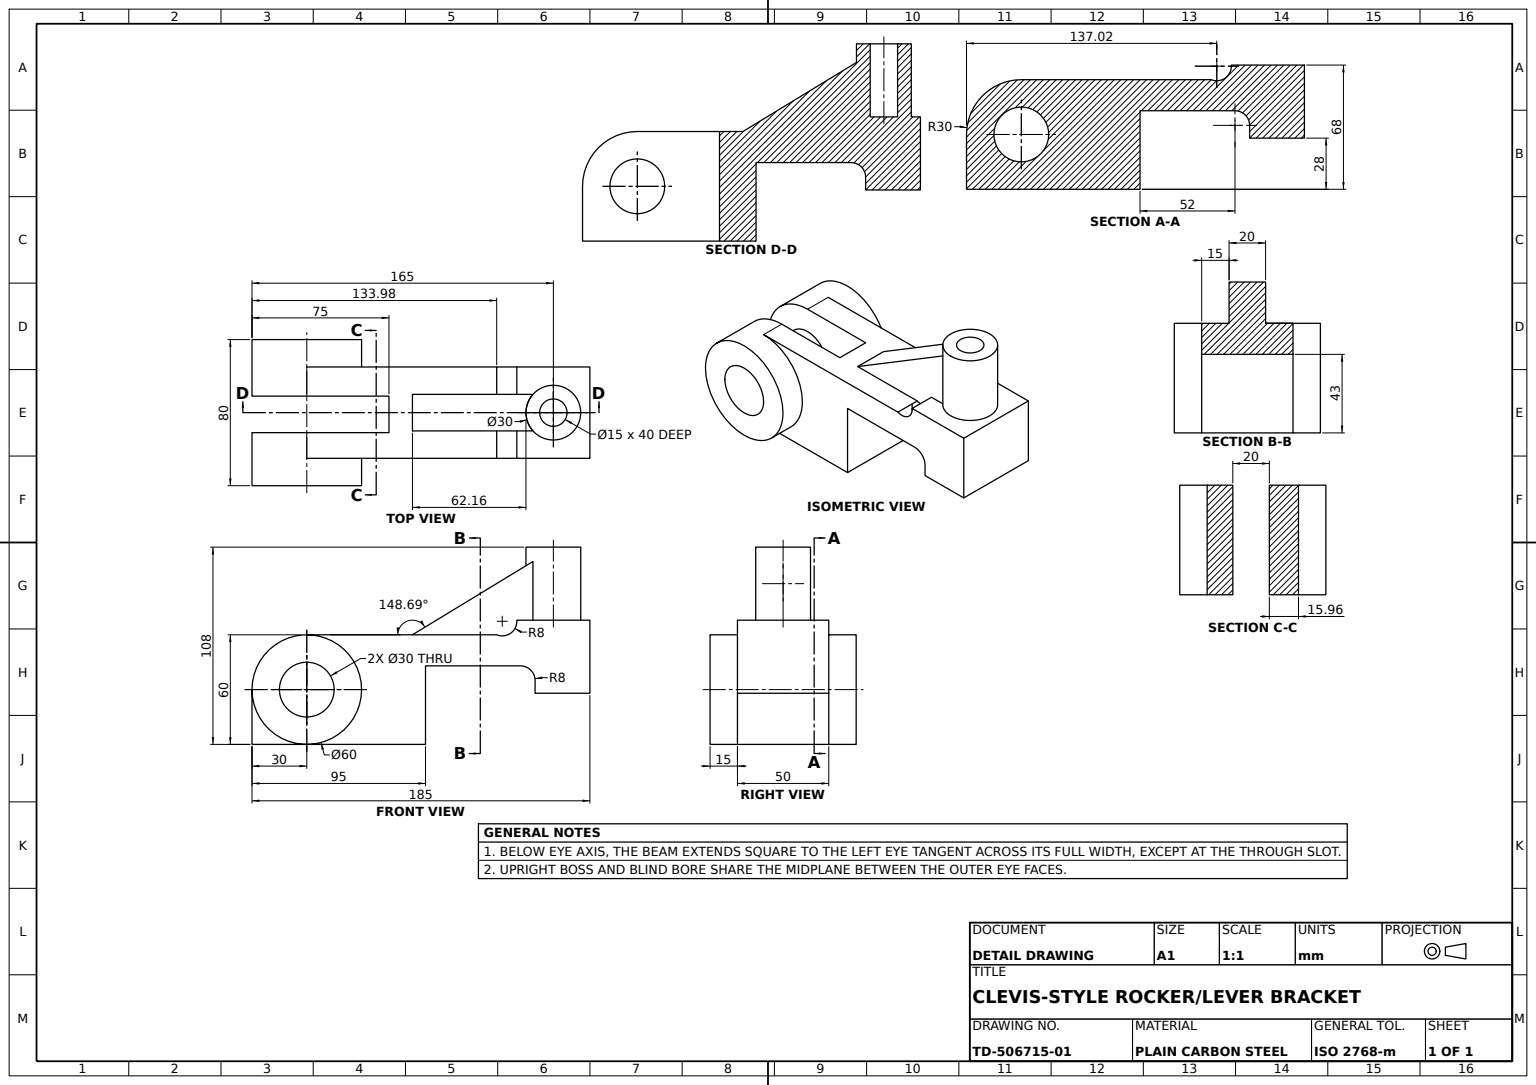
SolidWorks part; units mm, degrees
material "Plain Carbon Steel"
ref_plane "Front Plane" through (0, 0, 0) normal (0, 0, 1) x (1, 0, 0)
ref_plane "Top Plane" through (0, 0, 0) normal (0, 1, 0) x (1, 0, 0)
ref_plane "Right Plane" through (0, 0, 0) normal (1, 0, 0) x (0, 0, -1)
sketch "Arm Profile Sketch" plane through (0, 0, 0) normal (0, 0, 1) x (1, 0, 0)
  line L0 (0, 0) -> (30, 0)
  line L1 (30, 0) -> (30, 40)
  line L3 (0, 0) -> (0, 7)
  line L4 (-8, 15) -> (-60, 15)
  line L5 (-60, 15) -> (-60, -28)
  line L6 (-60, -28) -> (-155, -28)
  line L7 (-155, -28) -> (-155, 32)
  line L9 (-155, 32) -> (-21.0223, 32)
  line L11 (30, 40) -> (-10, 40)
  arc A0 (0, 7) -> (-8, 15) centre (-8, 7) ccw
  arc A2 (-10, 40) -> (-21.0223, 32) centre (-17.9773, 39.3979) cw
  dimension "D1" = 8
  dimension "D2" = 40
  dimension "D6" = 8
  dimension "D3" = 30
  dimension "D4" = 52
  dimension "D5" = 43
  dimension "D7" = 60
  dimension "D8" = 95
  dimension "D9" = 133.9777
  dimension "D10" = 137.0227
extrude "Arm Body" add sketch "Arm Profile Sketch" along normal blind 50
sketch "Front Lug Sketch" plane through (0, 0, 50) normal (0, 0, 1) x (1, 0, 0)
  line L0 (-21.0223, 32) -> (-155, 32) construction
  line L1 (-155, 32) -> (-155, -28) construction
  circle A0 centre (-125, 2) radius 15
  circle A1 centre (-125, 2) radius 30
  dimension "D1" = 30
  dimension "D3" = 30
  dimension "D4" = 60
  dimension "D2" = 30
extrude "Front Lug Ø30" add sketch "Front Lug Sketch" along normal blind 15
sketch "Rear Lug Sketch" plane through (0, 0, 0) normal (0, 0, -1) x (-1, 0, 0)
  line L0 (155, 32) -> (155, -28) construction
  line L1 (21.0223, 32) -> (155, 32) construction
  circle A0 centre (125, 2) radius 15
  circle A1 centre (125, 2) radius 30
  dimension "D1" = 30
  dimension "D2" = 60
  dimension "D3" = 30
  dimension "D4" = 30
extrude "Rear Lug Ø30" add sketch "Rear Lug Sketch" along normal blind 15
sketch "Top Slot Sketch" plane through (0, 32, 0) normal (0, 1, 0) x (1, 0, 0)
  line L0 (-21.0223, 0) -> (-125, 0) construction
  line L1 (-155, -15.9553) -> (-80, -15.9553)
  line L2 (-155, -15.9553) -> (-155, -35.9553)
  line L3 (-155, -35.9553) -> (-80, -35.9553)
  line L4 (-80, -15.9553) -> (-80, -35.9553)
  line L5 (-155, -15.9553) -> (-80, -35.9553) construction
  line L6 (-155, -35.9553) -> (-80, -15.9553) construction
  line L7 (-155, -50) -> (-155, 0) construction
  point P0 (-155, -25)
  dimension "D1" = 20
  dimension "D2" = 75
  dimension "D3" = 15.9553
  dimension "D4" = 25
extrude "Top Slot Cut" cut sketch "Top Slot Sketch" against normal through all
sketch "Lug Relief Sketch" plane through (0, 0, 50) normal (0, 0, 1) x (1, 0, 0)
  line L0 (-155, 32) -> (-125, 32)
  line L1 (-155, 32) -> (-155, 2)
  circle A0 centre (-125, 2) radius 30 construction
  arc A1 (-125, 32) -> (-155, 2) centre (-125, 2) ccw construction
  arc A2 (-155, 2) -> (-125, 32) centre (-125, 2) cw
extrude "Lug Relief Cut" cut sketch "Lug Relief Sketch" against normal through all
sketch "Pin Post Sketch" plane through (0, 40, 0) normal (0, 1, 0) x (1, 0, 0)
  line L0 (-10, -50) -> (-10, 0) construction
  line L1 (30, 0) -> (-10, 0) construction
  circle A0 centre (10, -25) radius 7.5
  circle A1 centre (10, -25) radius 15
  dimension "D1" = 15
  dimension "D2" = 30
  dimension "D3" = 20
  dimension "D4" = 25
extrude "Pin Post Ø15" add sketch "Pin Post Sketch" along normal blind 40
ref_plane "Rib Plane" through (0, 0, 25) normal (0, 0, 1) x (1, 0, 0)
sketch "Support Rib Sketch" plane through (0, 0, 25) normal (0, 0, 1) x (1, 0, 0)
  line L0 (-5, 69.8014) -> (-67.1552, 32)
  line L1 (-5, 80) -> (-5, 40) construction
  line L2 (-21.0223, 32) -> (-125, 32) construction
  dimension "D1" = 62.1552
  dimension "D2" = 37.8014
rib "Support Rib" sketch "Support Rib Sketch" sketch "Support Rib Sketch" thickness 20 extrusion direction parallel to sketch draft on no parameters "D1"=20
sketch "Eye Bore Sketch" plane through (0, 0, 50) normal (0, 0, 1) x (1, 0, 0)
  circle A0 centre (-125, 2) radius 15
  dimension "D1" = 30
extrude "Eye Bore" cut sketch "Eye Bore Sketch" against normal through all
